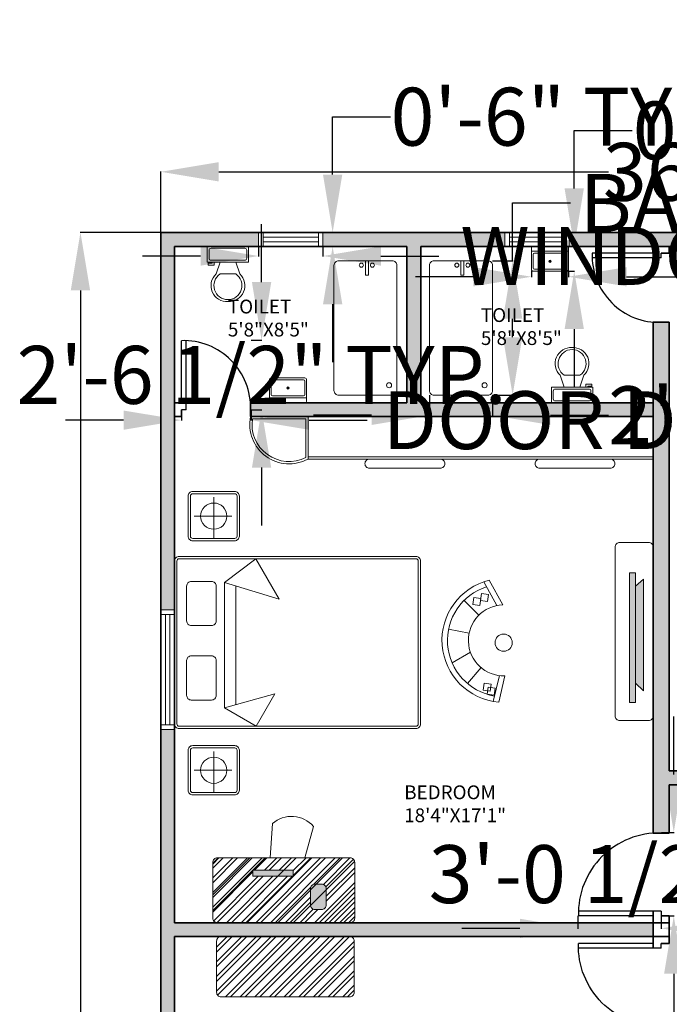
# Model space of a CAD drawing. Units: inches. Extents: x 35 to 5908, y 4 to 3165.
# Tile 4 of 6: x 4987 to 5270, y 2706 to 3134. Entities that reach past the tile are written whole.
import ezdxf

# ---------------------------------------------------------------- set-up
doc = ezdxf.new("R2010")
doc.units = ezdxf.units.IN
doc.header["$MEASUREMENT"] = 0
for name, color, linetype, lineweight in [('A-ANNO-DIMS', 2, 'Continuous', 18), ('A-DOOR', 4, 'Continuous', 25), ('A-FLOR-CASE', 8, 'Continuous', 18), ('A-FLOR-FIXT', 8, 'Continuous', 18), ('A-FURN', 8, 'Continuous', 18), ('A-FURN-PATT', 9, 'Continuous', 13), ('A-WALL', 7, 'Continuous', 35), ('A-WALL-PATT', 252, 'Continuous', 13)]:
    doc.layers.add(name, color=color, linetype=linetype, lineweight=lineweight)
doc.layers.add('A-AREA-IDEN', color=30, linetype='Continuous', lineweight=18, true_color=0xf8991e)
doc.layers.add('A-GLAZ', color=30, linetype='Continuous', lineweight=18, true_color=0xf8991e)
doc.styles.get("Standard").update_dxf_attribs({"font": 'arial.ttf'})
doc.dimstyles.get("Standard").update_dxf_attribs({"dimtxt": 25.18, "dimasz": 25.18, "dimexe": 0.18, "dimexo": 0.0625, "dimgap": 0.09, "dimtad": 0, "dimtih": 1, "dimtoh": 1, "dimdec": 0, "dimzin": 0, "dimdsep": 46, "dimlunit": 3, "dimtxsty": 'Standard', "dimcen": 0.09, "dimadec": 0, "dimazin": 0, "dimtfac": 1, "dimtdec": 0, "dimtofl": 0, "dimtmove": 0, "dimatfit": 3, "dimfxl": 1, "dimtolj": 1, "dimtzin": 0, "dimarcsym": 0})

# ---------------------------------------------------------------- blocks, each defined once
blk = doc.blocks.new('*U4')
for p, q in [((9.5, -6), (9.5, -2)), ((-10, -8.5), (-8, -8.5)), ((-10, -9.5), (-10, -8.5)), ((-7, -9.5), (-10, -9.5)), ((-8, -8.5), (-8, -8)), ((-7, -8), (-7, -9.5)), ((-4, -8), (-6, -14)), ((4, -8), (6, -14)), ((4, -14), (-4, -14))]:
    blk.add_line(p, q)
blk.add_lwpolyline([(10.5, -8), (10.5, 0), (-10.5, 0), (-10.5, -8)], close=True)
for points in [[(-9.5, -2), (-9.5, -6)], [(8.5, -1), (-8.5, -1)], [(-8.5, -7), (8.5, -7)]]:
    blk.add_lwpolyline(points)
for centre, radius, start, end in [((-8.625, -1.875), 0.8839, 81.8699, 188.1301), ((8.625, -1.875), 0.8839, 351.8699, 98.1301), ((-8.625, -6.125), 0.8839, 171.869898, 278.1301), ((8.625, -6.125), 0.8839, 261.8699, 8.1301), ((-0.4772, -19.9188), 8.0953, 133.01722, 273.38), ((0.0374, -19.8731), 7.127, 124.50543, 269.7), ((-0.0373, -19.8731), 7.127, 270.3, 55.4946), ((0.4773, -19.9188), 8.0953, 266.62, 46.9828)]:
    blk.add_arc(centre, radius, start, end)
blk = doc.blocks.new('Sink-single - 30 in top')
blk.add_line((-15, -3.999996), (15, -3.999996))
for points in [[(-13.5, 0), (13.5, 0)], [(-15, -18.499996), (-15, -1.5)], [(-13.5, -17.499996), (-13.5, -6.499996)], [(-12.5, -5.499996), (12.5, -5.499996)], [(13.5, -6.499996), (13.5, -17.499996)], [(15, -1.5), (15, -18.499996)], [(13.5, -19.999996), (-13.5, -19.999996)], [(12.5, -18.499996), (-12.5, -18.499996)]]:
    blk.add_lwpolyline(points)
for radius in [1, 0.5]:
    blk.add_circle((0, -11.999996), radius)
for centre, radius, start, end in [((-13.5, -1.5), 1.5, 90, 180), ((-12.5, -6.499996), 1, 90, 180), ((12.5, -6.499996), 1, 0, 90), ((13.5, -1.5), 1.5, 0, 90), ((-13.5, -18.499996), 1.5, 180, 270), ((-12.5, -17.499996), 1, 180, 270), ((12.5, -17.499996), 1, 270, 0), ((13.5, -18.499996), 1.5, 270, 0)]:
    blk.add_arc(centre, radius, start, end)
blk = doc.blocks.new('*D6')
at = {"layer": 'A-ANNO-DIMS', "color": 0, "lineweight": -2, "transparency": 16777216}
for p, q in [((5048.79, 3041.84), (5048.79, 3068.36)), ((5073.97, 3068.18), (5243.35, 3068.18)), ((5455.61, 3068.18), (5286.24, 3068.18)), ((5480.79, 3041.84), (5480.79, 3068.36))]:
    blk.add_line(p, q, dxfattribs=at)
for points in [[(5073.97, 3072.38), (5073.97, 3063.99), (5048.79, 3068.18)], [(5455.61, 3072.38), (5455.61, 3063.99), (5480.79, 3068.18)]]:
    blk.add_solid(points, dxfattribs=at)
at = {"layer": 'Defpoints', "color": 0, "lineweight": -2, "transparency": 16777216}
for p in [(5480.79, 3068.18), (5048.79, 3041.78), (5480.79, 3041.78)]:
    blk.add_point(p, dxfattribs=at)
at = {"layer": 'A-ANNO-DIMS', "color": 0, "transparency": 16777216, "insert": (5264.79, 3068.18), "char_height": 25.18, "attachment_point": 5}
blk.add_mtext("\\A1;36'", dxfattribs=at)
blk = doc.blocks.new('*D7')
at = {"layer": 'A-ANNO-DIMS', "color": 0, "lineweight": -2, "transparency": 16777216}
for p, q in [((5048.73, 3041.84), (5013.71, 3041.84)), ((5013.89, 3016.66), (5013.89, 2694.76)), ((5013.89, 2346.96), (5013.89, 2668.86)), ((5048.73, 2321.78), (5013.71, 2321.78))]:
    blk.add_line(p, q, dxfattribs=at)
for points in [[(5009.69, 3016.66), (5018.09, 3016.66), (5013.89, 3041.84)], [(5009.69, 2346.96), (5018.09, 2346.96), (5013.89, 2321.78)]]:
    blk.add_solid(points, dxfattribs=at)
at = {"layer": 'Defpoints', "color": 0, "lineweight": -2, "transparency": 16777216}
for p in [(5048.79, 3041.84), (5013.89, 2321.78), (5048.79, 2321.78)]:
    blk.add_point(p, dxfattribs=at)
at = {"layer": 'A-ANNO-DIMS', "color": 0, "transparency": 16777216, "insert": (5013.89, 2681.81), "char_height": 25.18, "attachment_point": 5}
blk.add_mtext("\\A1;60'", dxfattribs=at)
blk = doc.blocks.new('DOOR-30-3_5-JAMB')
for p, q in [((-3.5, 0), (-30, 0)), ((0, -2), (-30, -2)), ((0, -2), (0, 0))]:
    blk.add_line(p, q)
blk.add_arc((-1, -1), 29.02, 178.0251, 271.9749)
blk = doc.blocks.new('DOOR-30-3-JAMB')
for p, q in [((-2, -27), (-2, 0)), ((0, -30), (0, 0)), ((0, -30), (-2, -30))]:
    blk.add_line(p, q)
blk.add_arc((-1, -29), 29.02, 358.0251, 91.9749)
blk = doc.blocks.new('DOOR-36')
for p, q in [((0, 2), (-36, 2)), ((0, 2), (0, 0)), ((-3.5, 0), (-36, 0))]:
    blk.add_line(p, q)
blk.add_arc((-1, 1), 35.01, 88.3634, 181.6366)
blk = doc.blocks.new('WINDOW-48')
for p, q in [((0, 0), (0, 6)), ((2, 0), (2, 6)), ((50, 0), (50, 6)), ((52, 0), (52, 6)), ((2, 4), (50, 4)), ((2, 2), (50, 2))]:
    blk.add_line(p, q)
blk = doc.blocks.new('WINDOW-24')
for p, q in [((0, 0), (0, 6)), ((2, 0), (2, 6)), ((26, 0), (26, 6)), ((28, 0), (28, 6)), ((2, 4), (26, 4)), ((2, 2), (26, 2))]:
    blk.add_line(p, q)
blk = doc.blocks.new('BATH-TUB-MIXER')
blk.add_lwpolyline([(27.36, 56.41, 0.414214), (25.36, 58.41), (2, 58.41, 0.414214), (0, 56.41), (0, 2, 0.414214), (2, 0), (25.36, 0, 0.414214), (27.36, 2)], format="xyb", close=True)
blk.add_lwpolyline([(13.68, 58.41), (13.68, 58.41), (14.93, 58.41), (14.93, 58.41), (14.93, 52.09), (14.93, 52.09), (13.68, 52.09), (13.68, 52.09)], close=True)
for centre, radius in [((11.89, 56.48), 0.882), ((16.69, 56.48), 0.882), ((23.94, 4.28), 1.11)]:
    blk.add_circle(centre, radius)
blk = doc.blocks.new('SEATING-SEMICIRCULAR')
for p, q in [((-8.61, 26.49), (-2.9, 16.18)), ((-6.26, 27.18), (-0.33, 16.47)), ((-10.8, 11.96), (-17.22, 18.38)), ((-15.03, 4.08), (-23.93, 5.87)), ((-14.47, -4.08), (-22.37, -8.78)), ((-9.84, -10.8), (-15.69, -17.74)), ((-4.52, -25.5), (-1.86, -14.3)), ((-2.14, -25.8), (0.56, -14.43))]:
    blk.add_line(p, q)
for points in [[(-9.61, 21.43), (-10.07, 18.38), (-7.03, 17.91), (-6.56, 20.96)], [(-12.99, 19.72), (-13.45, 16.67), (-10.4, 16.21), (-9.94, 19.26)], [(-8.44, -17.54), (-8.91, -20.58), (-5.86, -21.05), (-5.4, -18)], [(-6.7, -19.36), (-7.17, -22.4), (-4.12, -22.87), (-3.66, -19.82)]]:
    blk.add_lwpolyline(points, close=True)
blk.add_circle((0, 0), 3.73)
for radius, start, end in [(26.92, 103.6927, 265.1976), (24.53, 107.9155, 260.4199), (15.45, 91.6667, 271.6667)]:
    blk.add_arc((0.12, 1.02), radius, start, end)
blk = doc.blocks.new('*D24')
at = {"layer": 'A-ANNO-DIMS', "color": 0, "lineweight": -2, "transparency": 16777216}
for p, q in [((5184.7, 3022.57), (5159.52, 3022.57)), ((5209.88, 3024.93), (5209.88, 3022.39)), ((5226.05, 3024.93), (5226.05, 3022.39)), ((5251.23, 3022.57), (5276.41, 3022.57))]:
    blk.add_line(p, q, dxfattribs=at)
for points in [[(5184.7, 3026.76), (5184.7, 3018.37), (5209.88, 3022.57)], [(5251.23, 3026.76), (5251.23, 3018.37), (5226.05, 3022.57)]]:
    blk.add_solid(points, dxfattribs=at)
at = {"layer": 'Defpoints', "color": 0, "lineweight": -2, "transparency": 16777216}
for p in [(5209.88, 3024.99), (5226.05, 3024.99), (5226.05, 3022.57)]:
    blk.add_point(p, dxfattribs=at)
at = {"layer": 'A-ANNO-DIMS', "color": 0, "transparency": 16777216, "insert": (5410.36, 3022.57), "char_height": 25.18, "attachment_point": 5}
blk.add_mtext('\\A1;BASIN 1\'-4" TYP.', dxfattribs=at)
blk = doc.blocks.new('*D25')
at = {"layer": 'A-ANNO-DIMS', "color": 0, "lineweight": -2, "transparency": 16777216}
for p, q in [((5228.48, 3060.96), (5228.48, 3086.14)), ((5228.48, 3086.14), (5253.66, 3086.14)), ((5226.12, 3035.78), (5228.66, 3035.78)), ((5226.12, 3024.99), (5228.66, 3024.99)), ((5228.48, 2999.81), (5228.48, 2974.63))]:
    blk.add_line(p, q, dxfattribs=at)
for points in [[(5224.28, 3060.96), (5232.68, 3060.96), (5228.48, 3035.78)], [(5224.28, 2999.81), (5232.68, 2999.81), (5228.48, 3024.99)]]:
    blk.add_solid(points, dxfattribs=at)
at = {"layer": 'Defpoints', "color": 0, "lineweight": -2, "transparency": 16777216}
for p in [(5226.05, 3035.78), (5228.48, 3035.78), (5226.05, 3024.99)]:
    blk.add_point(p, dxfattribs=at)
at = {"layer": 'A-ANNO-DIMS', "color": 0, "transparency": 16777216, "insert": (5340.27, 3086.14), "char_height": 25.18, "attachment_point": 5}
blk.add_mtext('\\A1;0\'-11" TYP.', dxfattribs=at)
blk = doc.blocks.new('*D28')
at = {"layer": 'A-ANNO-DIMS', "color": 0, "lineweight": -2, "transparency": 16777216}
for p, q in [((5091.29, 3035.72), (5091.29, 3031.4)), ((5119.29, 3035.72), (5119.29, 3031.4)), ((5066.11, 3031.58), (5040.93, 3031.58)), ((5144.47, 3031.58), (5169.65, 3031.58))]:
    blk.add_line(p, q, dxfattribs=at)
for points in [[(5066.11, 3035.78), (5066.11, 3027.38), (5091.29, 3031.58)], [(5144.47, 3035.78), (5144.47, 3027.38), (5119.29, 3031.58)]]:
    blk.add_solid(points, dxfattribs=at)
at = {"layer": 'Defpoints', "color": 0, "lineweight": -2, "transparency": 16777216}
for p in [(5091.29, 3035.78), (5119.29, 3035.78), (5119.29, 3031.58)]:
    blk.add_point(p, dxfattribs=at)
at = {"layer": 'A-ANNO-DIMS', "color": 0, "transparency": 16777216, "insert": (5360.33, 3031.58), "char_height": 25.18, "attachment_point": 5}
blk.add_mtext('\\A1;WINDOW W2 2\'-4" TYP.', dxfattribs=at)
blk = doc.blocks.new('*D29')
at = {"layer": 'A-ANNO-DIMS', "color": 0, "lineweight": -2, "transparency": 16777216}
for p, q in [((5123.49, 3066.96), (5123.49, 3092.14)), ((5123.49, 3092.14), (5148.67, 3092.14)), ((5119.36, 3041.78), (5123.67, 3041.78)), ((5119.36, 3035.78), (5123.67, 3035.78)), ((5123.49, 3010.6), (5123.49, 2985.42))]:
    blk.add_line(p, q, dxfattribs=at)
for points in [[(5119.3, 3066.96), (5127.69, 3066.96), (5123.49, 3041.78)], [(5119.3, 3010.6), (5127.69, 3010.6), (5123.49, 3035.78)]]:
    blk.add_solid(points, dxfattribs=at)
at = {"layer": 'Defpoints', "color": 0, "lineweight": -2, "transparency": 16777216}
for p in [(5119.29, 3041.78), (5123.49, 3041.78), (5119.29, 3035.78)]:
    blk.add_point(p, dxfattribs=at)
at = {"layer": 'A-ANNO-DIMS', "color": 0, "transparency": 16777216, "insert": (5225.51, 3092.14), "char_height": 25.18, "attachment_point": 5}
blk.add_mtext('\\A1;0\'-6" TYP.', dxfattribs=at)
blk = doc.blocks.new('*D30')
at = {"layer": 'A-ANNO-DIMS', "color": 0, "lineweight": -2, "transparency": 16777216}
for p, q in [((5057.79, 2964.72), (5057.79, 2960.06)), ((5088.07, 2964.72), (5088.07, 2960.06)), ((5032.61, 2960.24), (5007.43, 2960.24)), ((5113.25, 2960.24), (5138.43, 2960.24))]:
    blk.add_line(p, q, dxfattribs=at)
for points in [[(5032.61, 2964.43), (5032.61, 2956.04), (5057.79, 2960.24)], [(5113.25, 2964.43), (5113.25, 2956.04), (5088.07, 2960.24)]]:
    blk.add_solid(points, dxfattribs=at)
at = {"layer": 'Defpoints', "color": 0, "lineweight": -2, "transparency": 16777216}
for p in [(5057.79, 2964.78), (5088.07, 2964.78), (5088.07, 2960.24)]:
    blk.add_point(p, dxfattribs=at)
at = {"layer": 'A-ANNO-DIMS', "color": 0, "transparency": 16777216, "insert": (5329, 2960.24), "char_height": 25.18, "attachment_point": 5}
blk.add_mtext('\\A1;DOOR D2 2\'-6 1/2" TYP.', dxfattribs=at)
blk = doc.blocks.new('*D31')
at = {"layer": 'A-ANNO-DIMS', "color": 0, "lineweight": -2, "transparency": 16777216}
for p, q in [((5092.61, 3020.24), (5092.61, 3045.42)), ((5088.13, 2995.06), (5092.79, 2995.06)), ((5088.13, 2964.78), (5092.79, 2964.78)), ((5092.61, 2939.6), (5092.61, 2914.42))]:
    blk.add_line(p, q, dxfattribs=at)
for points in [[(5088.42, 3020.24), (5096.81, 3020.24), (5092.61, 2995.06)], [(5088.42, 2939.6), (5096.81, 2939.6), (5092.61, 2964.78)]]:
    blk.add_solid(points, dxfattribs=at)
at = {"layer": 'Defpoints', "color": 0, "lineweight": -2, "transparency": 16777216}
for p in [(5088.07, 2995.06), (5092.61, 2995.06), (5088.07, 2964.78)]:
    blk.add_point(p, dxfattribs=at)
at = {"layer": 'A-ANNO-DIMS', "color": 0, "transparency": 16777216, "insert": (5092.61, 2979.92), "char_height": 25.18, "attachment_point": 5}
blk.add_mtext('\\A1;2\'-6 1/2" TYP.', dxfattribs=at)
blk = doc.blocks.new('*D32')
at = {"layer": 'A-ANNO-DIMS', "color": 0, "lineweight": -2, "transparency": 16777216}
for p, q in [((5230.02, 2744.72), (5230.02, 2739.16)), ((5266.29, 2744.72), (5266.29, 2739.16)), ((5204.84, 2739.34), (5179.66, 2739.34)), ((5291.47, 2739.34), (5316.65, 2739.34))]:
    blk.add_line(p, q, dxfattribs=at)
for points in [[(5204.84, 2743.53), (5204.84, 2735.14), (5230.02, 2739.34)], [(5291.47, 2743.53), (5291.47, 2735.14), (5266.29, 2739.34)]]:
    blk.add_solid(points, dxfattribs=at)
at = {"layer": 'Defpoints', "color": 0, "lineweight": -2, "transparency": 16777216}
for p in [(5230.02, 2744.78), (5266.29, 2744.78), (5266.29, 2739.34)]:
    blk.add_point(p, dxfattribs=at)
at = {"layer": 'A-ANNO-DIMS', "color": 0, "transparency": 16777216, "insert": (5507.22, 2739.34), "char_height": 25.18, "attachment_point": 5}
blk.add_mtext('\\A1;DOOR D3 3\'-0 1/2" TYP.', dxfattribs=at)
blk = doc.blocks.new('*D33')
at = {"layer": 'A-ANNO-DIMS', "color": 0, "lineweight": -2, "transparency": 16777216}
for p, q in [((5271.74, 2806.23), (5271.74, 2831.41)), ((5266.36, 2781.05), (5271.92, 2781.05)), ((5266.36, 2744.78), (5271.92, 2744.78)), ((5271.74, 2719.6), (5271.74, 2694.42))]:
    blk.add_line(p, q, dxfattribs=at)
for points in [[(5267.54, 2806.23), (5275.93, 2806.23), (5271.74, 2781.05)], [(5267.54, 2719.6), (5275.93, 2719.6), (5271.74, 2744.78)]]:
    blk.add_solid(points, dxfattribs=at)
at = {"layer": 'Defpoints', "color": 0, "lineweight": -2, "transparency": 16777216}
for p in [(5266.29, 2781.05), (5271.74, 2781.05), (5266.29, 2744.78)]:
    blk.add_point(p, dxfattribs=at)
at = {"layer": 'A-ANNO-DIMS', "color": 0, "transparency": 16777216, "insert": (5271.74, 2762.92), "char_height": 25.18, "attachment_point": 5}
blk.add_mtext('\\A1;3\'-0 1/2" TYP.', dxfattribs=at)
blk = doc.blocks.new('*D34')
at = {"layer": 'A-ANNO-DIMS', "color": 0, "lineweight": -2, "transparency": 16777216}
for p, q in [((5201.71, 3029.52), (5201.71, 3054.7)), ((5201.71, 3054.7), (5226.89, 3054.7)), ((5193.01, 3029.52), (5201.89, 3029.52)), ((5201.71, 2996.29), (5201.71, 3004.34)), ((5193.01, 2971.11), (5201.89, 2971.11))]:
    blk.add_line(p, q, dxfattribs=at)
for points in [[(5197.51, 3004.34), (5205.9, 3004.34), (5201.71, 3029.52)], [(5197.51, 2996.29), (5205.9, 2996.29), (5201.71, 2971.11)]]:
    blk.add_solid(points, dxfattribs=at)
at = {"layer": 'Defpoints', "color": 0, "lineweight": -2, "transparency": 16777216}
for p in [(5192.94, 3029.52), (5201.71, 3029.52), (5192.94, 2971.11)]:
    blk.add_point(p, dxfattribs=at)
at = {"layer": 'A-ANNO-DIMS', "color": 0, "transparency": 16777216, "insert": (5429.25, 3054.7), "char_height": 25.18, "attachment_point": 5}
blk.add_mtext('\\A1;BATHTUB 4\'-10 1/2" TYP.', dxfattribs=at)
blk = doc.blocks.new('*D35')
at = {"layer": 'A-ANNO-DIMS', "color": 0, "lineweight": -2, "transparency": 16777216}
for p, q in [((5165.59, 2971.05), (5165.59, 2962.17)), ((5192.94, 2971.05), (5192.94, 2962.17)), ((5140.41, 2962.35), (5115.23, 2962.35)), ((5218.12, 2962.35), (5243.3, 2962.35))]:
    blk.add_line(p, q, dxfattribs=at)
for points in [[(5140.41, 2966.54), (5140.41, 2958.15), (5165.59, 2962.35)], [(5218.12, 2966.54), (5218.12, 2958.15), (5192.94, 2962.35)]]:
    blk.add_solid(points, dxfattribs=at)
at = {"layer": 'Defpoints', "color": 0, "lineweight": -2, "transparency": 16777216}
for p in [(5165.59, 2971.11), (5192.94, 2971.11), (5192.94, 2962.35)]:
    blk.add_point(p, dxfattribs=at)
at = {"layer": 'A-ANNO-DIMS', "color": 0, "transparency": 16777216, "insert": (5349.69, 2962.35), "char_height": 25.18, "attachment_point": 5}
blk.add_mtext('\\A1;2\'-3 1/2" TYP.', dxfattribs=at)

msp = doc.modelspace()

# ---------------------------------------------------------------- hatches: boundary and pattern name
at = {"layer": 'A-FURN-PATT'}
h = msp.add_hatch(color=256, dxfattribs=at)
h.dxf.hatch_style = 1
h.paths.add_polyline_path([(5258.55, 2891.08), (5255.12, 2888.06), (5255.12, 2845.97), (5258.55, 2842.54)])
h.paths.add_polyline_path([(5255.12, 2893.9), (5252.5, 2893.9), (5252.5, 2837.51), (5255.12, 2837.51)])
h = msp.add_hatch(dxfattribs=at)
h.set_pattern_fill('ANSI32', color=256, scale=38)
h.paths.add_polyline_path([(5133.08, 2767.98, 0.414214), (5131.08, 2769.98), (5073.4, 2769.98, 0.414214), (5071.4, 2767.98), (5071.4, 2743.78, 0.414214), (5073.4, 2741.78), (5131.08, 2741.78, 0.414214), (5133.08, 2743.78)])
h = msp.add_hatch(dxfattribs=at)
h.set_pattern_fill('ANSI32', color=256, scale=12)
h.paths.add_polyline_path([(5132.89, 2733.78, 0.414214), (5130.89, 2735.78), (5075.06, 2735.78, 0.414214), (5073.06, 2733.78), (5073.06, 2711.55, 0.414214), (5075.06, 2709.55), (5130.89, 2709.55, 0.414214), (5132.89, 2711.55)])
h.paths.add_polyline_path([(5133.08, 2767.98, 0.414214), (5131.08, 2769.98), (5073.4, 2769.98, 0.414214), (5071.4, 2767.98), (5071.4, 2743.78, 0.414214), (5073.4, 2741.78), (5131.08, 2741.78, 0.414214), (5133.08, 2743.78)])
h.paths.add_polyline_path([(5088.87, 2761.97), (5088.87, 2764.61), (5106.39, 2764.61), (5106.39, 2761.97)], flags=16)
h.paths.add_polyline_path([(5113.86, 2756.62, -0.414214), (5115.86, 2758.62), (5118.68, 2758.62, -0.414214), (5120.68, 2756.62), (5120.68, 2749.55, -0.414214), (5118.68, 2747.55), (5115.86, 2747.55, -0.414214), (5113.86, 2749.55)], flags=16)
h = msp.add_hatch(color=256, dxfattribs=at)
h.dxf.hatch_style = 1
h.paths.add_polyline_path([(5106.39, 2764.61), (5088.87, 2764.61), (5088.87, 2761.97), (5106.39, 2761.97)])
h.paths.add_polyline_path([(5120.68, 2756.62, 0.414214), (5118.68, 2758.62), (5115.86, 2758.62, 0.414214), (5113.86, 2756.62), (5113.86, 2749.55, 0.414214), (5115.86, 2747.55), (5118.68, 2747.55, 0.414214), (5120.68, 2749.55)])
at = {"layer": 'A-WALL-PATT'}
h = msp.add_hatch(color=256, dxfattribs=at)
h.dxf.hatch_style = 1
h.paths.add_polyline_path([(5198.29, 3041.78), (5119.29, 3041.78), (5119.29, 3035.78), (5155.79, 3035.78), (5155.79, 2967.78), (5087.79, 2967.78), (5087.79, 2966.78, -0.017236), (5087.79, 2964.78), (5087.79, 2961.78), (5262.79, 2961.78), (5262.79, 2967.78), (5236.55, 2967.78), (5236.55, 2967.75), (5218.53, 2967.75), (5161.79, 2967.78), (5161.79, 3035.78), (5198.29, 3035.78)])
h.paths.add_polyline_path([(5091.29, 3041.78), (5048.79, 3041.78), (5048.79, 2877.78), (5054.79, 2877.78), (5054.79, 2899), (5054.79, 2961.78), (5054.79, 2967.78), (5054.79, 3035.78), (5091.29, 3035.78)])
h.paths.add_polyline_path([(5346.29, 3041.78), (5226.29, 3041.78), (5226.29, 3035.78), (5262.79, 3035.78), (5269.79, 3035.78), (5346.29, 3035.78)])
h.paths.add_polyline_path([(5480.79, 3041.78), (5398.29, 3041.78), (5398.29, 3035.78), (5407.91, 3035.78), (5474.79, 3035.78), (5474.79, 2807.78), (5269.79, 2807.78), (5269.79, 3002.78), (5266.29, 3002.78, -0.017236), (5264.29, 3002.78), (5262.79, 3002.78), (5262.79, 2967.78), (5262.79, 2961.78), (5262.79, 2780.78), (5264.29, 2780.78, -0.014283), (5266.29, 2780.78), (5269.79, 2780.78), (5269.79, 2801.78), (5412.79, 2801.78), (5412.79, 2712.78), (5346.79, 2712.78), (5346.79, 2706.78), (5421.79, 2706.78), (5421.79, 2709.78, -0.017236), (5421.79, 2711.78), (5421.79, 2712.78), (5418.79, 2712.78), (5418.79, 2801.78), (5474.79, 2801.78), (5474.79, 2712.78), (5454.79, 2712.78), (5454.79, 2706.78), (5474.79, 2706.78), (5474.79, 2668.42), (5480.79, 2668.42)])
h.paths.add_polyline_path([(5054.79, 2825.78), (5048.79, 2825.78), (5048.79, 2632.28), (5054.79, 2632.28), (5054.79, 2642.69), (5054.79, 2735.78), (5262.79, 2735.78), (5262.79, 2741.78), (5054.79, 2741.78)])
h.paths.add_polyline_path([(5480.79, 2616.42), (5474.79, 2616.42), (5474.79, 2502.2), (5480.79, 2502.2)])
h.paths.add_polyline_path([(5407.53, 2562.78), (5269.79, 2562.78), (5269.79, 2696.78), (5266.29, 2696.78, -0.014283), (5264.29, 2696.78), (5262.79, 2696.78), (5262.79, 2509.78), (5264.29, 2509.78, -0.017236), (5266.29, 2509.78), (5269.79, 2509.78), (5269.79, 2556.78), (5407.53, 2556.78)])
h.paths.add_polyline_path([(5262.79, 2530.78), (5087.79, 2530.78), (5087.79, 2527.78, -0.017236), (5087.79, 2525.78), (5087.79, 2524.78), (5143.79, 2524.78), (5143.79, 2514.78), (5149.79, 2514.78), (5149.79, 2524.78), (5171.79, 2524.78), (5171.79, 2514.78), (5177.79, 2514.78), (5177.79, 2524.78), (5262.79, 2524.78)], flags=17)
h.paths.add_polyline_path([(5262.79, 2395.71), (5262.79, 2321.78), (5480.79, 2321.78), (5480.79, 2450.2), (5474.79, 2450.2), (5474.79, 2381.78), (5425.29, 2381.78), (5425.29, 2375.78), (5474.79, 2375.78), (5474.79, 2327.78), (5269.79, 2327.78), (5269.79, 2375.78), (5312.61, 2375.78), (5312.61, 2381.78), (5269.79, 2381.78), (5269.79, 2395.71)])
h.paths.add_polyline_path([(5171.13, 2321.78), (5171.13, 2327.78), (5054.79, 2327.78), (5054.79, 2470.78), (5157.79, 2470.78), (5262.79, 2470.78), (5262.79, 2461.71), (5269.79, 2461.71), (5269.79, 2476.78), (5262.79, 2476.78), (5177.79, 2476.78), (5177.79, 2486.78), (5171.79, 2486.78), (5171.79, 2476.78), (5149.79, 2476.78), (5149.79, 2486.78), (5143.79, 2486.78), (5143.79, 2476.78), (5054.79, 2476.78), (5054.79, 2580.28), (5048.79, 2580.28), (5048.79, 2321.78)])

# ---------------------------------------------------------------- linework, layer by layer
at = {"layer": 'A-FLOR-CASE'}
for p, q in [((5112.84, 2943.34), (5112.84, 2961.78)), ((5088.63, 2960.78), (5111.84, 2960.78)), ((5111.84, 2943.94), (5111.84, 2960.78)), ((5262.79, 2944.34), (5112.84, 2944.34)), ((5262.79, 2943.34), (5112.84, 2943.34))]:
    msp.add_line(p, q, dxfattribs=at)
for points in [[(5137.53, 2941.34, -0.414214), (5139.53, 2943.34), (5170.23, 2943.34, -0.414214), (5172.23, 2941.34), (5172.23, 2941.3, -0.414214), (5170.23, 2939.3), (5139.53, 2939.3, -0.414214), (5137.53, 2941.3)], [(5211.49, 2941.34, -0.414214), (5213.49, 2943.34), (5244.18, 2943.34, -0.414214), (5246.18, 2941.34), (5246.18, 2941.3, -0.414214), (5244.18, 2939.3), (5213.49, 2939.3, -0.414214), (5211.49, 2941.3)]]:
    msp.add_lwpolyline(points, format="xyb", close=True, dxfattribs=at)
for radius, start, end in [(17.14, 168.4994, 298.7732), (16.14, 171.3861, 296.6929)]:
    msp.add_arc((5104.59, 2958.36), radius, start, end, dxfattribs=at)
at = {"layer": 'A-FURN'}
for p, q in [((5071.82, 2918.52), (5071.82, 2926.72)), ((5071.82, 2926.72), (5071.82, 2908.81)), ((5063.28, 2918.52), (5079.74, 2918.52)), ((5076.53, 2889.65), (5090.12, 2900)), ((5090.12, 2900), (5100.24, 2882.47)), ((5076.53, 2835.25), (5076.53, 2889.65)), ((5100.24, 2882.47), (5076.53, 2889.65)), ((5255.12, 2888.06), (5258.55, 2891.08)), ((5258.55, 2891.08), (5258.55, 2842.54)), ((5081.39, 2888.18), (5081.36, 2836.57)), ((5258.55, 2842.54), (5255.12, 2845.97)), ((5098.41, 2841.21), (5076.53, 2835.25)), ((5090.33, 2827.2), (5098.41, 2841.21)), ((5076.53, 2835.25), (5090.33, 2827.2)), ((5071.82, 2808.07), (5071.82, 2816.27)), ((5071.82, 2816.27), (5071.82, 2798.36)), ((5063.28, 2808.07), (5079.74, 2808.07)), ((5096.39, 2769.98), (5097.38, 2784.85)), ((5115.12, 2783.67), (5111.41, 2769.98))]:
    msp.add_line(p, q, dxfattribs=at)
for points in [[(5060.69, 2927.23, -0.414214), (5062.69, 2929.23), (5080.95, 2929.23, -0.414214), (5082.95, 2927.23), (5082.95, 2909.81, -0.414214), (5080.95, 2907.81), (5062.69, 2907.81, -0.414214), (5060.69, 2909.81)], [(5061.69, 2927.23, -0.414214), (5062.69, 2928.23), (5080.95, 2928.23, -0.414214), (5081.95, 2927.23), (5081.95, 2909.81, -0.414214), (5080.95, 2908.81), (5062.69, 2908.81, -0.414214), (5061.69, 2909.81)], [(5262.79, 2905.04, 0.414214), (5260.79, 2907.04), (5248.28, 2907.04, 0.414214), (5246.28, 2905.04), (5246.28, 2831.68, 0.414214), (5248.28, 2829.68), (5260.79, 2829.68, 0.414214), (5262.79, 2831.68)], [(5054.79, 2899, -0.414214), (5056.79, 2901), (5159.71, 2901, -0.414214), (5161.71, 2899), (5161.71, 2828.2, -0.414214), (5159.71, 2826.2), (5056.79, 2826.2, -0.414214), (5054.79, 2828.2)], [(5055.79, 2899, -0.414214), (5056.79, 2900), (5159.71, 2900, -0.414214), (5160.71, 2899), (5160.71, 2828.2, -0.414214), (5159.71, 2827.2), (5056.79, 2827.2, -0.414214), (5055.79, 2828.2)], [(5060.05, 2888.13, -0.414214), (5062.05, 2890.13), (5070.86, 2890.13, -0.414214), (5072.86, 2888.13), (5072.86, 2872.95, -0.414214), (5070.86, 2870.95), (5062.05, 2870.95, -0.414214), (5060.05, 2872.95)], [(5060.05, 2855.77, -0.414214), (5062.05, 2857.77), (5070.86, 2857.77, -0.414214), (5072.86, 2855.77), (5072.86, 2840.59, -0.414214), (5070.86, 2838.59), (5062.05, 2838.59, -0.414214), (5060.05, 2840.59)], [(5060.69, 2816.77, -0.414214), (5062.69, 2818.77), (5080.95, 2818.77, -0.414214), (5082.95, 2816.77), (5082.95, 2799.36, -0.414214), (5080.95, 2797.36), (5062.69, 2797.36, -0.414214), (5060.69, 2799.36)], [(5061.69, 2816.77, -0.414214), (5062.69, 2817.77), (5080.95, 2817.77, -0.414214), (5081.95, 2816.77), (5081.95, 2799.36, -0.414214), (5080.95, 2798.36), (5062.69, 2798.36, -0.414214), (5061.69, 2799.36)], [(5071.4, 2743.78, 0.414214), (5073.4, 2741.78), (5131.08, 2741.78, 0.414214), (5133.08, 2743.78), (5133.08, 2767.98, 0.414214), (5131.08, 2769.98), (5073.4, 2769.98, 0.414214), (5071.4, 2767.98)], [(5113.86, 2756.62, -0.414214), (5115.86, 2758.62), (5118.68, 2758.62, -0.414214), (5120.68, 2756.62), (5120.68, 2749.55, -0.414214), (5118.68, 2747.55), (5115.86, 2747.55, -0.414214), (5113.86, 2749.55)], [(5073.06, 2733.78, -0.414214), (5075.06, 2735.78), (5130.89, 2735.78, -0.414214), (5132.89, 2733.78), (5132.89, 2711.55, -0.414214), (5130.89, 2709.55), (5075.06, 2709.55, -0.414214), (5073.06, 2711.55)]]:
    msp.add_lwpolyline(points, format="xyb", close=True, dxfattribs=at)
for points in [[(5252.5, 2893.9), (5252.5, 2893.9), (5255.12, 2893.9), (5255.12, 2893.9), (5255.12, 2837.51), (5255.12, 2837.51), (5252.5, 2837.51), (5252.5, 2837.51)], [(5088.87, 2764.61), (5088.87, 2764.61), (5106.39, 2764.61), (5106.39, 2764.61), (5106.39, 2761.97), (5106.39, 2761.97), (5088.87, 2761.97), (5088.87, 2761.97)]]:
    msp.add_lwpolyline(points, close=True, dxfattribs=at)
for centre in [(5071.82, 2918.52), (5071.82, 2808.07)]:
    msp.add_circle(centre, 5.7, dxfattribs=at)
msp.add_arc((5105.68, 2775.66), 12.38, 40.3188, 132.0414, dxfattribs=at)
at = {"layer": 'A-WALL'}
for p, q in [((5048.79, 2321.78), (5048.79, 3041.78)), ((5048.79, 3041.78), (5480.79, 3041.78)), ((5054.79, 3035.78), (5155.79, 3035.78)), ((5054.79, 2967.78), (5054.79, 3035.78)), ((5155.79, 2967.78), (5155.79, 3035.78)), ((5161.79, 2967.78), (5161.79, 3035.78)), ((5161.79, 3035.78), (5262.79, 3035.78)), ((5262.79, 3035.78), (5269.79, 3035.78)), ((5262.79, 3030.78), (5262.79, 3035.78)), ((5269.79, 3035.78), (5269.79, 3032.78)), ((5269.79, 3035.78), (5474.79, 3035.78)), ((5266.29, 3032.78), (5269.79, 3032.78)), ((5262.79, 2967.78), (5262.79, 3002.87)), ((5262.79, 3002.78), (5269.79, 3002.78)), ((5269.79, 3002.78), (5269.79, 2807.78)), ((5054.79, 2967.78), (5059.79, 2967.78)), ((5054.79, 2967.78), (5054.79, 2961.78)), ((5087.74, 2967.78), (5155.79, 2967.78)), ((5087.79, 2967.78), (5087.79, 2961.78)), ((5161.79, 2967.78), (5262.79, 2967.78)), ((5262.79, 2780.7), (5262.79, 2967.78)), ((5054.79, 2961.78), (5057.79, 2961.78)), ((5054.79, 2741.78), (5054.79, 2961.78)), ((5057.79, 2964.78), (5057.79, 2961.78)), ((5087.79, 2961.78), (5262.79, 2961.78)), ((5269.79, 2807.78), (5474.79, 2807.78)), ((5269.79, 2801.78), (5412.79, 2801.78)), ((5269.79, 2801.78), (5269.79, 2780.78)), ((5262.79, 2780.78), (5269.79, 2780.78)), ((5262.79, 2730.78), (5262.79, 2746.78)), ((5266.29, 2744.78), (5269.79, 2744.78)), ((5269.79, 2744.78), (5269.79, 2732.78)), ((5054.79, 2741.78), (5262.79, 2741.78)), ((5262.79, 2741.78), (5269.79, 2741.78)), ((5054.79, 2735.78), (5262.79, 2735.78)), ((5054.79, 2476.78), (5054.79, 2735.78)), ((5262.79, 2735.78), (5269.79, 2735.78)), ((5266.29, 2732.78), (5269.79, 2732.78))]:
    msp.add_line(p, q, dxfattribs=at)

# ---------------------------------------------------------------- block references
at = {"layer": 'A-DOOR'}
for name, p in [('DOOR-30-3_5-JAMB', (5266.29, 3032.78)), ('DOOR-30-3-JAMB', (5059.79, 2994.78)), ('DOOR-36', (5266.29, 2744.78))]:
    msp.add_blockref(name, p, dxfattribs=at)
at = {"layer": 'A-DOOR', "extrusion": (0, 0, -1), "zscale": -1, "rotation": 180}
msp.add_blockref('DOOR-36', (-5266.29, 2732.78), dxfattribs=at)
at = {"layer": 'A-FLOR-FIXT'}
for name, p, xscale, yscale, zscale in [('*U4', (5077.98, 3035.78), 0.8581878397813429, 0.8581878397813429, 0.8581878397813429), ('Sink-single - 30 in top', (5217.96, 3035.78), 0.5392550146415948, 0.5392550146415948, 0.5392550146415948)]:
    msp.add_blockref(name, p, dxfattribs=dict(at, xscale=xscale, yscale=yscale, zscale=zscale))
for p in [(5124.08, 2971.11), (5165.58, 2971.11)]:
    msp.add_blockref('BATH-TUB-MIXER', p, dxfattribs=at)
at = {"layer": 'A-FLOR-FIXT', "rotation": 180}
for name, p, xscale, yscale, zscale in [('*U4', (5227.54, 2967.75), 0.8581878397813429, 0.8581878397813429, 0.8581878397813429), ('Sink-single - 30 in top', (5104.07, 2967.78), 0.5392550146415948, 0.5392550146415948, 0.5392550146415948)]:
    msp.add_blockref(name, p, dxfattribs=dict(at, xscale=xscale, yscale=yscale, zscale=zscale))
at = {"layer": 'A-FURN'}
msp.add_blockref('SEATING-SEMICIRCULAR', (5197.81, 2863.5), dxfattribs=at)
at = {"layer": 'A-GLAZ'}
msp.add_blockref('WINDOW-24', (5091.3, 3035.78), dxfattribs=at)
for name, p, rotation in [('WINDOW-24', (5226.29, 3041.78), 180), ('WINDOW-48', (5054.79, 2825.78), 89.99999999999991)]:
    msp.add_blockref(name, p, dxfattribs=dict(at, rotation=rotation))

# ---------------------------------------------------------------- texts
at = {"layer": 'A-AREA-IDEN', "char_height": 6, "attachment_point": 1}
for s, insert in [('TOILET\\P5\'8"X8\'5"', (5077.98, 3012.61)), ('TOILET\\P5\'8"X8\'5"', (5187.92, 3008.91)), ('BEDROOM\\P18\'4"X17\'1"', (5154.59, 2801.48))]:
    msp.add_mtext_dynamic_manual_height_columns(s, width=69.8687, gutter_width=1, heights=[0], dxfattribs=dict(at, insert=insert))

# ---------------------------------------------------------------- dimensions: what is measured, and where the dimension line sits
at = {"layer": 'A-ANNO-DIMS'}
for base, p1, p2, text, picture, middle in [((5201.71, 3029.52), (5192.94, 2971.11), (5192.94, 3029.52), 'BATHTUB <> TYP.', '*D34', (5429.25, 3054.7)), ((5123.49, 3041.78), (5119.29, 3035.78), (5119.29, 3041.78), '<> TYP.', '*D29', (5225.51, 3092.14)), ((5228.48, 3035.78), (5226.05, 3024.99), (5226.05, 3035.78), '<> TYP.', '*D25', (5340.27, 3086.14)), ((5092.61, 2995.06), (5088.07, 2964.78), (5088.07, 2995.06), '<> TYP.', '*D31', (5092.61, 2979.92)), ((5271.74, 2781.05), (5266.29, 2744.78), (5266.29, 2781.05), '<> TYP.', '*D33', (5271.74, 2762.92))]:
    dim = msp.add_linear_dim(base=base, p1=p1, p2=p2, angle=90, text=text, dimstyle='Standard', override={"dimdec": 1, "dimlfac": 1, "dimrnd": 0, "dimzin": 1, "dimdsep": 46, "dimlunit": 4, "dimfrac": 2}, dxfattribs=at)
    dim.commit()
    dim.dimension.update_dxf_attribs({"geometry": picture, "text_midpoint": middle})
for base, p1, p2, text, picture, middle in [((5119.29, 3031.58), (5091.29, 3035.78), (5119.29, 3035.78), 'WINDOW W2 <> TYP.', '*D28', (5360.33, 3031.58)), ((5226.05, 3022.57), (5209.88, 3024.99), (5226.05, 3024.99), 'BASIN <> TYP.', '*D24', (5410.36, 3022.57)), ((5088.07, 2960.24), (5057.79, 2964.78), (5088.07, 2964.78), 'DOOR D2 <> TYP.', '*D30', (5329, 2960.24)), ((5192.9443, 2962.3472), (5165.5853, 2971.109), (5192.9443, 2971.109), '<> TYP.', '*D35', (5349.6879, 2962.3472)), ((5266.29, 2739.34), (5230.02, 2744.78), (5266.29, 2744.78), 'DOOR D3 <> TYP.', '*D32', (5507.22, 2739.34))]:
    dim = msp.add_linear_dim(base=base, p1=p1, p2=p2, text=text, dimstyle='Standard', override={"dimdec": 1, "dimlfac": 1, "dimrnd": 0, "dimzin": 1, "dimdsep": 46, "dimlunit": 4, "dimfrac": 2}, dxfattribs=at)
    dim.commit()
    dim.dimension.update_dxf_attribs({"geometry": picture, "text_midpoint": middle})
dim = msp.add_linear_dim(base=(5480.79, 3068.18), p1=(5048.79, 3041.78), p2=(5480.79, 3041.78), dimstyle='Standard', override={"dimclrd": 0, "dimclre": 0, "dimclrt": 0}, dxfattribs=at)
dim.commit()
dim.dimension.update_dxf_attribs({"geometry": '*D6', "text_midpoint": (5264.79, 3068.18)})
dim = msp.add_linear_dim(base=(5013.89, 2321.78), p1=(5048.79, 3041.84), p2=(5048.79, 2321.78), angle=90, dimstyle='Standard', override={"dimclrd": 0, "dimclre": 0, "dimclrt": 0}, dxfattribs=at)
dim.commit()
dim.dimension.update_dxf_attribs({"geometry": '*D7', "text_midpoint": (5013.89, 2681.81)})

doc.saveas('drawing.dxf')
